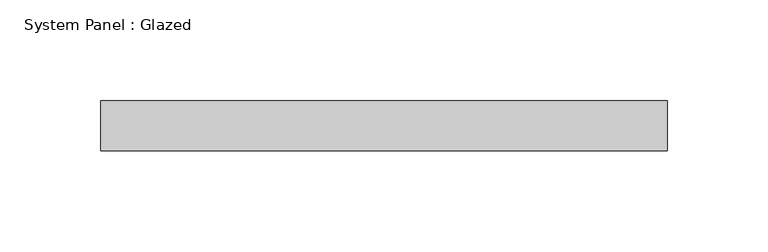
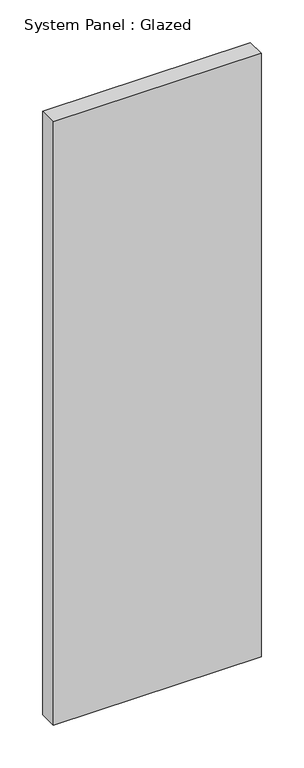
"""IFC4 building model written with IfcOpenShell, lengths in millimetres: plate geometry, System Panel : Glazed."""

from ifc_helpers import new_model, si_unit, origin, origin_with_axes, place, context, project, spatial, polyline, outline, extrude, source, transform, mapped, element, save


def system_panel_glazed_703d63a0(model_context):
    return source(origin(), model_context, "Body", "SweptSolid", [
        extrude(outline(polyline([(140.7583333, 24.5), (-140.7583333, 24.5), (-140.7583333, 49.5), (140.7583333, 49.5), (140.7583333, 24.5)])), origin_with_axes(), (0.0, 0.0, 1.0), 864.4),
    ])


if __name__ == "__main__":
    model = new_model("IFC4")
    model_context = context("Model", 3, world=origin())
    ifc_project = project(units=[si_unit("LENGTHUNIT", "METRE", prefix="MILLI")], contexts=[model_context])
    site = spatial("IfcSite", under=ifc_project)
    building = spatial("IfcBuilding", under=site)
    placement = place(None, origin())
    system_panel_glazed_shape = system_panel_glazed_703d63a0(model_context)
    element("IfcPlate", 1, ObjectType="System Panel : Glazed", at=placement, inside=building, context=model_context, shape_type="MappedRepresentation", body=[
        mapped(system_panel_glazed_shape, transform((0.0, 0.0, 0.0), x_axis=(1.0, 0.0, 0.0), y_axis=(0.0, 1.0, 0.0), z_axis=(0.0, 0.0, 1.0))),
    ])
    save(model, "model.ifc")

# Revit data of these elements
# Type "System Panel : Glazed"
#   Keynote = "H11"
#   Construction Type Id = "GSP4R"
#   Analytic Construction = "1/8 in Pilkington single glazing"
#   Visual Light Transmittance = 0.9
#   Solar Heat Gain Coefficient = 0.86
#   Heat Transfer Coefficient (U) = 6.7069 W/(m²·K)
#   Define Thermal Properties by = 1
# Element 1 (IfcPlate, "System Panel : Glazed")
#   Materials on its faces: "Glass"
# Materials
#   "Glass": class "Glass", colour RGB 0 128 192, transparency 0.9, Description = "Soda Lime Glass", Cost = 0
